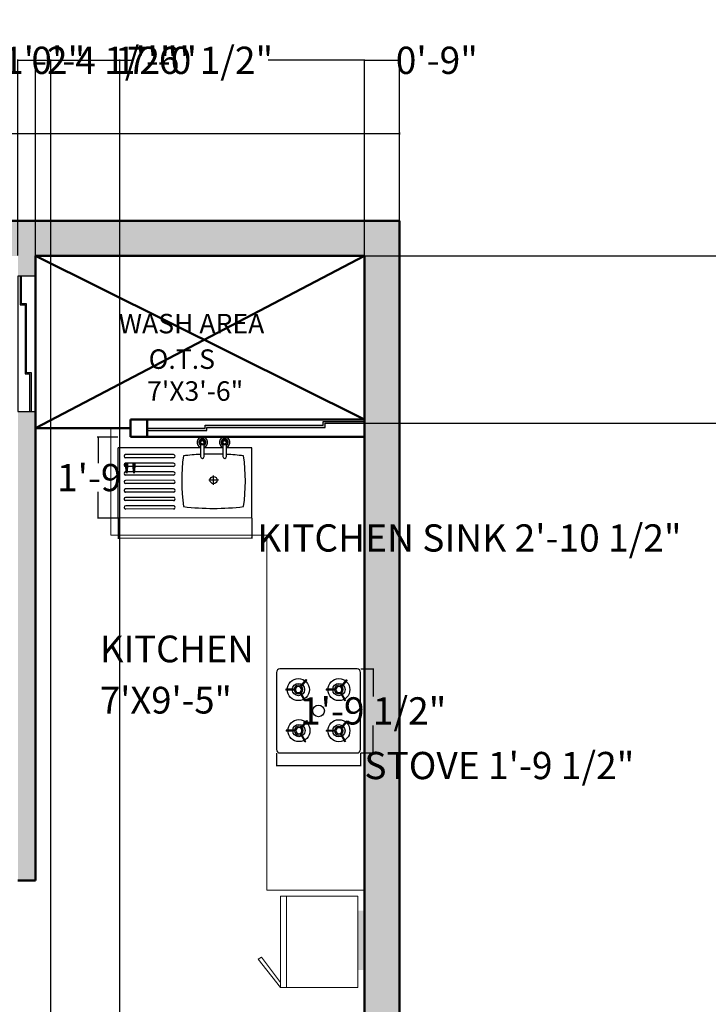
# Model space of a CAD drawing. Units: inches. Extents: x 48 to 822, y -191 to 651.
# Tile 8 of 13: x 268 to 445, y 398 to 651. Entities that reach past the tile are written whole.
import ezdxf

# ---------------------------------------------------------------- set-up
doc = ezdxf.new("R2010")
doc.units = ezdxf.units.IN
doc.header["$MEASUREMENT"] = 0
doc.layers.get('0').update_dxf_attribs({"color": 254})
for name, color, linetype, lineweight in [('A-ANNO-DIMS', 2, 'Continuous', 18), ('A-AREA-IDEN', 7, 'Continuous', 25), ('A-FLOR-FIXT', 8, 'Continuous', 18), ('A-FURN', 8, 'Continuous', 18), ('A-GLAZ', 4, 'Continuous', 25), ('A-WALL', 7, 'Continuous', 50), ('A-WALL-PATT', 8, 'Continuous', 13)]:
    doc.layers.add(name, color=color, linetype=linetype, lineweight=lineweight)
doc.layers.add('furniture', color=250, linetype='Continuous')
doc.styles.get("Standard").update_dxf_attribs({"font": 'arial.ttf'})
doc.dimstyles.get("Standard").update_dxf_attribs({"dimtxt": 7, "dimasz": 0.18, "dimexe": 0.18, "dimexo": 0.0625, "dimgap": 0.09, "dimtad": 0, "dimtih": 1, "dimtoh": 1, "dimzin": 0, "dimdsep": 46, "dimlunit": 3, "dimtxsty": 'Standard', "dimcen": 0.09, "dimadec": 0, "dimazin": 0, "dimtfac": 1, "dimtofl": 0, "dimtmove": 0, "dimatfit": 3, "dimfxl": 1, "dimtolj": 1, "dimtzin": 0, "dimarcsym": 0})

# ---------------------------------------------------------------- blocks, each defined once
blk = doc.blocks.new('4bstove')
at = {"layer": 'furniture'}
for p, q in [((1452.73, 1446.21), (1452.73, 1448.61)), ((1452.98, 1446.22), (1452.98, 1448.61)), ((1464.44, 1446.34), (1464.44, 1448.73)), ((1464.69, 1446.34), (1464.69, 1448.73)), ((1451.74, 1444.45), (1449.67, 1443.25)), ((1451.87, 1444.23), (1449.79, 1443.04)), ((1453.75, 1444.08), (1455.58, 1442.54)), ((1453.91, 1444.27), (1455.74, 1442.73)), ((1463.45, 1444.58), (1461.38, 1443.38)), ((1463.57, 1444.36), (1461.5, 1443.17)), ((1465.46, 1444.21), (1467.29, 1442.67)), ((1465.62, 1444.4), (1467.45, 1442.86)), ((1452.69, 1434.81), (1452.69, 1437.2)), ((1452.94, 1434.81), (1452.94, 1437.2)), ((1464.44, 1434.81), (1464.44, 1437.2)), ((1464.69, 1434.81), (1464.69, 1437.2)), ((1451.7, 1433.04), (1449.63, 1431.85)), ((1451.82, 1432.83), (1449.75, 1431.63)), ((1453.71, 1432.67), (1455.54, 1431.13)), ((1453.87, 1432.86), (1455.7, 1431.33)), ((1463.45, 1433.04), (1461.38, 1431.85)), ((1463.57, 1432.83), (1461.5, 1431.63)), ((1465.46, 1432.67), (1467.29, 1431.13)), ((1465.62, 1432.86), (1467.45, 1431.33))]:
    blk.add_line(p, q, dxfattribs=at)
for points in [[(1447.5, 1427.38), (1469.5, 1427.38, 0.414214), (1470.5, 1428.38), (1470.5, 1450.38, 0.414214), (1469.5, 1451.38), (1447.5, 1451.38, 0.414214), (1446.5, 1450.38), (1446.5, 1428.38, 0.414214)], [(1453.75, 1444.97, 1), (1452, 1444.97, 1)], [(1465.46, 1445.1, 1), (1463.71, 1445.1, 1)], [(1453.71, 1433.56, 1), (1451.96, 1433.56, 1)], [(1465.46, 1433.56, 1), (1463.71, 1433.56, 1)]]:
    blk.add_lwpolyline(points, format="xyb", close=True, dxfattribs=at)
for points in [[(1454.12, 1444.97, 1), (1451.62, 1444.97, 1), (1454.12, 1444.97, 1)], [(1465.83, 1445.1, 1), (1463.33, 1445.1, 1), (1465.83, 1445.1, 1)], [(1454.08, 1433.56, 1), (1451.58, 1433.56, 1), (1454.08, 1433.56, 1)], [(1465.83, 1433.56, 1), (1463.33, 1433.56, 1), (1465.83, 1433.56, 1)]]:
    blk.add_lwpolyline(points, format="xyb", dxfattribs=at)
for centre, radius in [((1452.87, 1444.97), 3.14), ((1464.58, 1445.1), 3.14), ((1452.87, 1444.97), 1.75), ((1464.58, 1445.1), 1.75), ((1458.5, 1439.38), 1.67), ((1452.83, 1433.56), 3.14), ((1464.58, 1433.56), 3.14), ((1452.83, 1433.56), 1.75), ((1464.58, 1433.56), 1.75)]:
    blk.add_circle(centre, radius, dxfattribs=at)
for centre, start, end in [((1452.87, 1444.97), 88.2645, 92.2039), ((1464.58, 1445.1), 88.2645, 92.2039), ((1452.87, 1444.97), 208.188, 212.1274), ((1452.87, 1444.97), 318.1018, 322.0412), ((1464.58, 1445.1), 208.188, 212.1274), ((1464.58, 1445.1), 318.1018, 322.0412), ((1452.83, 1433.56), 88.2645, 92.2039), ((1464.58, 1433.56), 88.2645, 92.2039)]:
    blk.add_arc(centre, 3.64, start, end, dxfattribs=at)
blk = doc.blocks.new('stove')
at = {"layer": 'furniture', "xscale": 0.9, "yscale": 0.9, "zscale": 0.9, "rotation": 89.99999999999999}
blk.add_blockref('4bstove', (1295.44, -1312.65), dxfattribs=at)
blk = doc.blocks.new('A$C799204C7')
for p, q in [((0, 34.2), (17.99, 34.2)), ((0, 0), (0, 34.2)), ((17.99, 13.08), (17.99, 34.2)), ((2.32, 20.01), (2.32, 32.27)), ((3.13, 20.01), (3.13, 32.27)), ((4.48, 20.01), (4.48, 32.27)), ((5.29, 20.01), (5.29, 32.27)), ((6.64, 20.01), (6.64, 32.27)), ((7.45, 20.01), (7.45, 32.27)), ((8.85, 20.01), (8.85, 32.27)), ((9.66, 20.01), (9.66, 32.27)), ((11.01, 20.01), (11.01, 32.27)), ((11.82, 20.01), (11.82, 32.27)), ((13.22, 20.01), (13.22, 32.27)), ((14.03, 20.01), (14.03, 32.27)), ((15.42, 20.01), (15.42, 32.27)), ((16.24, 20.01), (16.24, 32.27)), ((18.59, 13.08), (15.71, 13.08)), ((9.73, 11), (9.73, 8.54)), ((15.71, 12.17), (18.59, 12.17)), ((17.99, 7.36), (17.99, 12.17)), ((8.52, 9.77), (10.9, 9.77)), ((18.59, 7.36), (15.71, 7.36)), ((15.71, 6.45), (18.59, 6.45)), ((17.99, 0), (17.99, 6.45)), ((0, 0), (17.99, 0))]:
    blk.add_line(p, q)
for centre, radius in [((19.38, 12.62), 0.684), ((19.38, 12.62), 0.456), ((9.7, 9.77), 0.916), ((19.38, 6.91), 0.684), ((19.38, 6.91), 0.456)]:
    blk.add_circle(centre, radius)
for centre, radius, start, end in [((2.72, 32.27), 0.407, 0, 180), ((4.88, 32.27), 0.407, 0, 180), ((7.05, 32.27), 0.407, 0, 180), ((9.25, 32.27), 0.407, 0, 180), ((11.42, 32.27), 0.407, 0, 180), ((13.62, 32.27), 0.407, 0, 180), ((15.83, 32.27), 0.407, 0, 180), ((2.72, 20.01), 0.407, 180, 0), ((9.53, -30.19), 48.1, 82.3437, 97.8966), ((4.88, 20.01), 0.407, 180, 0), ((7.05, 20.01), 0.407, 180, 0), ((9.25, 20.01), 0.407, 180, 0), ((11.42, 20.01), 0.407, 180, 0), ((13.62, 20.01), 0.407, 180, 0), ((15.83, 20.01), 0.407, 180, 0), ((67.33, 9.77), 64.88, 173.1952, 186.8048), ((-48.51, 9.77), 64.88, 2.9208, 6.8048), ((15.71, 12.62), 0.456, 90, 270), ((19.38, 12.62), 1.37, 199.6514, 160.3603), ((19.38, 12.62), 0.911, 210.3431, 149.7554), ((-48.51, 9.77), 64.88, 357.8723, 2.115), ((19.38, 6.91), 1.37, 199.6514, 160.3603), ((19.38, 6.91), 0.911, 210.3431, 149.7554), ((15.71, 6.91), 0.456, 90, 270), ((-48.51, 9.77), 64.88, 353.1952, 357.0665), ((9.53, 49.73), 48.1, 262.1034, 277.6563)]:
    blk.add_arc(centre, radius, start, end)
blk = doc.blocks.new('sink')
at = {"layer": 'furniture'}
for p, q in [((8718164203.894819, -1433730582.369047), (8718164201.504578, -1433730582.369047)), ((8718164202.684322, -1433730581.131674), (8718164202.684322, -1433730583.598095)), ((8718164196.150837, -1433730592.638258), (8718164196.150837, -1433730604.938997)), ((8718164196.967728, -1433730592.638258), (8718164196.967728, -1433730604.938997)), ((8718164198.365185, -1433730592.638258), (8718164198.365185, -1433730604.938997)), ((8718164199.182076, -1433730592.638258), (8718164199.182076, -1433730604.938997)), ((8718164200.579533, -1433730592.638258), (8718164200.579533, -1433730604.938997)), ((8718164201.396423, -1433730592.638258), (8718164201.396423, -1433730604.938997)), ((8718164202.748692, -1433730592.638258), (8718164202.748692, -1433730604.938997)), ((8718164203.565582, -1433730592.638258), (8718164203.565582, -1433730604.938997)), ((8718164204.963041, -1433730592.638258), (8718164204.963041, -1433730604.938997)), ((8718164205.779934, -1433730592.638258), (8718164205.779934, -1433730604.938997)), ((8718164207.1322, -1433730592.638258), (8718164207.1322, -1433730604.938997)), ((8718164207.949093, -1433730592.638258), (8718164207.949093, -1433730604.938997)), ((8718164209.301359, -1433730592.638258), (8718164209.301359, -1433730604.938997)), ((8718164210.118252, -1433730592.638258), (8718164210.118252, -1433730604.938997))]:
    blk.add_line(p, q, dxfattribs=at)
for centre, radius in [((8718164192.998869, -1433730579.495552), 0.685789), ((8718164192.998869, -1433730579.495552), 0.457192), ((8718164202.715019, -1433730582.369047), 0.919003), ((8718164192.998869, -1433730585.228166), 0.68579), ((8718164192.998869, -1433730585.228166), 0.68579), ((8718164192.998869, -1433730585.228166), 0.457192)]:
    blk.add_circle(centre, radius, dxfattribs=at)
for centre, radius, start, end in [((8718164196.559284, -1433730592.638258), 0.41045, 354.3355999, 185.6644001), ((8718164198.77363, -1433730592.638258), 0.41045, 354.3355999, 185.6644001), ((8718164200.98798, -1433730592.638258), 0.41045, 354.3355999, 185.6644001), ((8718164203.157139, -1433730592.638258), 0.41045, 354.3355999, 185.6644001), ((8718164205.371487, -1433730592.638258), 0.41045, 354.3355999, 185.6644001), ((8718164207.540646, -1433730592.640262), 0.41045, 354.3355999, 185.6644001), ((8718164209.709805, -1433730592.640262), 0.41045, 354.3355999, 185.6644001), ((8718164196.559284, -1433730604.938997), 0.408445, 180, 0), ((8718164198.77363, -1433730604.938997), 0.408445, 180, 0), ((8718164200.98798, -1433730604.938997), 0.408445, 180, 0), ((8718164203.157139, -1433730604.938997), 0.408445, 180, 0), ((8718164205.371487, -1433730604.938997), 0.408445, 180, 0), ((8718164207.540646, -1433730604.938997), 0.408445, 180, 0), ((8718164209.709805, -1433730604.938997), 0.408445, 180, 0)]:
    blk.add_arc(centre, radius, start, end, dxfattribs=at)
at = {"layer": 'furniture', "xscale": 1.0032, "yscale": 1.0032, "zscale": 1.0032, "rotation": 180}
blk.add_blockref('A$C799204C7', (8718164212.441259, -1433730572.566334), dxfattribs=at)
blk = doc.blocks.new('washbasin')
at = {"layer": 'furniture'}
blk.add_blockref('sink', (-8718164214.119328, 1433730589.721069), dxfattribs=at)
blk = doc.blocks.new('*D16')
at = {"layer": 'A-ANNO-DIMS', "color": 0, "lineweight": -2, "transparency": 16777216}
for p, q in [((125.45, 622.39), (125.45, 621.91)), ((365.45, 622.39), (365.45, 621.91)), ((125.63, 622.09), (239.36, 622.09)), ((365.27, 622.09), (251.54, 622.09))]:
    blk.add_line(p, q, dxfattribs=at)
at = {"layer": 'A-ANNO-DIMS', "color": 0, "transparency": 16777216}
for points in [[(125.63, 622.12), (125.63, 622.06), (125.45, 622.09)], [(365.27, 622.12), (365.27, 622.06), (365.45, 622.09)]]:
    blk.add_solid(points, dxfattribs=at)
at = {"layer": 'Defpoints', "color": 0, "transparency": 16777216}
for p in [(125.45, 622.45), (365.45, 622.45), (365.45, 622.09)]:
    blk.add_point(p, dxfattribs=at)
at = {"layer": 'A-ANNO-DIMS', "color": 0, "transparency": 16777216, "insert": (245.45, 622.09), "char_height": 7, "attachment_point": 5}
blk.add_mtext("\\A1;20'", dxfattribs=at)
blk = doc.blocks.new('WIN-1500')
for p, q in [((300.62, 546.44), (315.51, 546.44)), ((315.51, 546.44), (315.51, 547.24)), ((315.51, 547.24), (345.84, 547.24)), ((315.95, 545.8), (315.95, 546.59)), ((315.95, 546.59), (346.31, 546.59)), ((345.84, 547.24), (345.84, 548.17)), ((345.84, 548.17), (356.45, 548.17)), ((346.31, 546.59), (346.31, 547.73)), ((346.31, 547.73), (356.45, 547.73)), ((300.62, 545.8), (315.95, 545.8))]:
    blk.add_line(p, q)
blk = doc.blocks.new('WIN-900-SLIT')
for p, q in [((271.95, 585.52), (267.45, 585.52)), ((267.45, 585.52), (267.45, 550.72)), ((268.05, 585.52), (268.05, 578.13)), ((268.38, 578.41), (268.38, 585.52)), ((271.95, 550.72), (271.95, 585.52)), ((268.05, 578.13), (269.28, 578.13)), ((269.63, 578.41), (268.38, 578.41)), ((269.28, 578.13), (269.28, 560.35)), ((269.63, 560.61), (269.63, 578.41)), ((269.28, 560.35), (270.46, 560.35)), ((270.92, 560.61), (269.63, 560.61)), ((270.46, 560.35), (270.46, 550.72)), ((270.92, 550.72), (270.92, 560.61)), ((267.45, 550.72), (271.95, 550.72))]:
    blk.add_line(p, q)
blk = doc.blocks.new('*D54')
at = {"layer": 'A-ANNO-DIMS', "color": 0, "lineweight": -2, "transparency": 16777216}
for p, q in [((333.84, 462.92), (333.84, 459.57)), ((355.44, 462.92), (355.44, 459.57)), ((334.02, 459.75), (355.26, 459.75)), ((355.44, 459.75), (355.62, 459.75))]:
    blk.add_line(p, q, dxfattribs=at)
at = {"layer": 'A-ANNO-DIMS', "color": 0, "transparency": 16777216}
for points in [[(334.02, 459.78), (334.02, 459.72), (333.84, 459.75)], [(355.26, 459.78), (355.26, 459.72), (355.44, 459.75)]]:
    blk.add_solid(points, dxfattribs=at)
at = {"layer": 'Defpoints', "color": 0, "transparency": 16777216}
for p in [(333.84, 462.99), (355.44, 462.99), (355.44, 459.75)]:
    blk.add_point(p, dxfattribs=at)
at = {"layer": 'A-ANNO-DIMS', "color": 0, "transparency": 16777216, "insert": (391.08, 459.75), "char_height": 7, "attachment_point": 5}
blk.add_mtext('\\A1;STOVE 1\'-9 1/2"', dxfattribs=at)
blk = doc.blocks.new('*D55')
at = {"layer": 'A-ANNO-DIMS', "color": 0, "lineweight": -2, "transparency": 16777216}
for p, q in [((355.5, 484.59), (358.86, 484.59)), ((358.68, 484.41), (358.68, 477.49)), ((358.68, 463.17), (358.68, 470.08)), ((355.5, 462.99), (358.86, 462.99))]:
    blk.add_line(p, q, dxfattribs=at)
at = {"layer": 'A-ANNO-DIMS', "color": 0, "transparency": 16777216}
for points in [[(358.65, 484.41), (358.71, 484.41), (358.68, 484.59)], [(358.65, 463.17), (358.71, 463.17), (358.68, 462.99)]]:
    blk.add_solid(points, dxfattribs=at)
at = {"layer": 'Defpoints', "color": 0, "transparency": 16777216}
for p in [(355.44, 484.59), (358.68, 484.59), (355.44, 462.99)]:
    blk.add_point(p, dxfattribs=at)
at = {"layer": 'A-ANNO-DIMS', "color": 0, "transparency": 16777216, "insert": (358.68, 473.79), "char_height": 7, "attachment_point": 5}
blk.add_mtext('\\A1;1\'-9 1/2"', dxfattribs=at)
blk = doc.blocks.new('*D58')
at = {"layer": 'A-ANNO-DIMS', "color": 0, "lineweight": -2, "transparency": 16777216}
for p, q in [((293.18, 523.27), (293.19, 518.01)), ((327.49, 523.3), (327.5, 518.04)), ((293.37, 518.19), (327.32, 518.22)), ((327.5, 518.22), (327.68, 518.22))]:
    blk.add_line(p, q, dxfattribs=at)
at = {"layer": 'A-ANNO-DIMS', "color": 0, "transparency": 16777216}
for points in [[(293.37, 518.22), (293.37, 518.16), (293.19, 518.19)], [(327.32, 518.25), (327.32, 518.19), (327.5, 518.22)]]:
    blk.add_solid(points, dxfattribs=at)
at = {"layer": 'Defpoints', "color": 0, "transparency": 16777216}
for p in [(293.18, 523.33), (327.49, 523.36), (327.5, 518.22)]:
    blk.add_point(p, dxfattribs=at)
at = {"layer": 'A-ANNO-DIMS', "color": 0, "transparency": 16777216, "insert": (383.38, 518.22), "char_height": 7, "attachment_point": 5}
blk.add_mtext('\\A1;KITCHEN SINK 2\'-10 1/2"', dxfattribs=at)
blk = doc.blocks.new('*D59')
at = {"layer": 'A-ANNO-DIMS', "color": 0, "lineweight": -2, "transparency": 16777216}
for p, q in [((293.1, 544.15), (287.84, 544.14)), ((288.02, 543.96), (288.03, 537.4)), ((288.04, 523.51), (288.03, 530.07)), ((293.12, 523.33), (287.86, 523.33))]:
    blk.add_line(p, q, dxfattribs=at)
at = {"layer": 'A-ANNO-DIMS', "color": 0, "transparency": 16777216}
for points in [[(288.05, 543.96), (287.99, 543.96), (288.02, 544.14)], [(288.07, 523.51), (288.01, 523.51), (288.04, 523.33)]]:
    blk.add_solid(points, dxfattribs=at)
at = {"layer": 'Defpoints', "color": 0, "transparency": 16777216}
for p in [(293.17, 544.15), (288.04, 523.33), (293.18, 523.33)]:
    blk.add_point(p, dxfattribs=at)
at = {"layer": 'A-ANNO-DIMS', "color": 0, "transparency": 16777216, "insert": (288.03, 533.73), "char_height": 7, "attachment_point": 5}
blk.add_mtext('\\A1;1\'-9"', dxfattribs=at)
blk = doc.blocks.new('*D62')
at = {"layer": 'A-ANNO-DIMS', "color": 0, "lineweight": -2, "transparency": 16777216}
for p, q in [((267.45, 590.75), (267.45, 641.12)), ((267.63, 640.94), (271.77, 640.94)), ((271.95, 590.75), (271.95, 641.12)), ((271.95, 640.94), (272.13, 640.94))]:
    blk.add_line(p, q, dxfattribs=at)
at = {"layer": 'A-ANNO-DIMS', "color": 0, "transparency": 16777216}
for points in [[(267.63, 640.97), (267.63, 640.91), (267.45, 640.94)], [(271.77, 640.97), (271.77, 640.91), (271.95, 640.94)]]:
    blk.add_solid(points, dxfattribs=at)
at = {"layer": 'Defpoints', "color": 0, "transparency": 16777216}
for p in [(271.95, 640.94), (267.45, 590.69), (271.95, 590.69)]:
    blk.add_point(p, dxfattribs=at)
at = {"layer": 'A-ANNO-DIMS', "color": 0, "transparency": 16777216, "insert": (289.68, 640.94), "char_height": 7, "attachment_point": 5}
blk.add_mtext('\\A1;0\'-4 1/2"', dxfattribs=at)
blk = doc.blocks.new('*D63')
at = {"layer": 'A-ANNO-DIMS', "color": 0, "lineweight": -2, "transparency": 16777216}
for p, q in [((271.95, 590.75), (271.95, 641.12)), ((272.13, 640.94), (296.68, 640.94)), ((356.27, 640.94), (331.72, 640.94)), ((356.45, 590.75), (356.45, 641.12))]:
    blk.add_line(p, q, dxfattribs=at)
at = {"layer": 'A-ANNO-DIMS', "color": 0, "transparency": 16777216}
for points in [[(272.13, 640.97), (272.13, 640.91), (271.95, 640.94)], [(356.27, 640.97), (356.27, 640.91), (356.45, 640.94)]]:
    blk.add_solid(points, dxfattribs=at)
at = {"layer": 'Defpoints', "color": 0, "transparency": 16777216}
for p in [(356.45, 640.94), (271.95, 590.69), (356.45, 590.69)]:
    blk.add_point(p, dxfattribs=at)
at = {"layer": 'A-ANNO-DIMS', "color": 0, "transparency": 16777216, "insert": (314.2, 640.94), "char_height": 7, "attachment_point": 5}
blk.add_mtext('\\A1;7\'-0 1/2"', dxfattribs=at)
blk = doc.blocks.new('*D64')
at = {"layer": 'A-ANNO-DIMS', "color": 0, "lineweight": -2, "transparency": 16777216}
for p, q in [((356.45, 590.75), (356.45, 641.12)), ((356.63, 640.94), (365.27, 640.94)), ((365.45, 599.75), (365.45, 641.12)), ((365.45, 640.94), (365.63, 640.94))]:
    blk.add_line(p, q, dxfattribs=at)
at = {"layer": 'A-ANNO-DIMS', "color": 0, "transparency": 16777216}
for points in [[(356.63, 640.97), (356.63, 640.91), (356.45, 640.94)], [(365.27, 640.97), (365.27, 640.91), (365.45, 640.94)]]:
    blk.add_solid(points, dxfattribs=at)
at = {"layer": 'Defpoints', "color": 0, "transparency": 16777216}
for p in [(365.45, 640.94), (365.45, 599.69), (356.45, 590.69)]:
    blk.add_point(p, dxfattribs=at)
at = {"layer": 'A-ANNO-DIMS', "color": 0, "transparency": 16777216, "insert": (375.02, 640.94), "char_height": 7, "attachment_point": 5}
blk.add_mtext('\\A1;0\'-9"', dxfattribs=at)
blk = doc.blocks.new('*D84')
at = {"layer": 'A-ANNO-DIMS', "color": 0, "lineweight": -2, "transparency": 16777216}
for p, q in [((356.51, 590.69), (790.04, 590.69)), ((789.86, 590.51), (789.86, 572.87)), ((789.86, 547.91), (789.86, 565.54)), ((356.51, 547.73), (790.04, 547.73))]:
    blk.add_line(p, q, dxfattribs=at)
at = {"layer": 'A-ANNO-DIMS', "color": 0, "transparency": 16777216}
for points in [[(789.83, 590.51), (789.89, 590.51), (789.86, 590.69)], [(789.83, 547.91), (789.89, 547.91), (789.86, 547.73)]]:
    blk.add_solid(points, dxfattribs=at)
at = {"layer": 'Defpoints', "color": 0, "transparency": 16777216}
for p in [(356.45, 590.69), (356.45, 547.73), (789.86, 547.73)]:
    blk.add_point(p, dxfattribs=at)
at = {"layer": 'A-ANNO-DIMS', "color": 0, "transparency": 16777216, "insert": (789.86, 569.21), "char_height": 7, "attachment_point": 5}
blk.add_mtext('\\A1;3\'-7"', dxfattribs=at)
blk = doc.blocks.new('*D90')
at = {"layer": 'A-ANNO-DIMS', "color": 0, "lineweight": -2, "transparency": 16777216}
for p, q in [((250.94, 295.25), (250.94, 641.12)), ((251.12, 640.94), (264.75, 640.94)), ((264.93, 295.25), (264.93, 641.12)), ((264.93, 640.94), (265.11, 640.94))]:
    blk.add_line(p, q, dxfattribs=at)
at = {"layer": 'A-ANNO-DIMS', "color": 0, "transparency": 16777216}
for points in [[(251.12, 640.97), (251.12, 640.91), (250.94, 640.94)], [(264.75, 640.97), (264.75, 640.91), (264.93, 640.94)]]:
    blk.add_solid(points, dxfattribs=at)
at = {"layer": 'Defpoints', "color": 0, "transparency": 16777216}
for p in [(264.93, 640.94), (250.94, 295.19), (264.93, 295.19)]:
    blk.add_point(p, dxfattribs=at)
at = {"layer": 'A-ANNO-DIMS', "color": 0, "transparency": 16777216, "insert": (274.17, 640.94), "char_height": 7, "attachment_point": 5}
blk.add_mtext('\\A1;1\'-2"', dxfattribs=at)
blk = doc.blocks.new('*D92')
at = {"layer": 'A-ANNO-DIMS', "color": 0, "lineweight": -2, "transparency": 16777216}
for p, q in [((275.91, 79.24), (275.91, 641.12)), ((276.09, 640.94), (293.48, 640.94)), ((293.66, 79.24), (293.66, 641.12)), ((293.66, 640.94), (293.84, 640.94))]:
    blk.add_line(p, q, dxfattribs=at)
at = {"layer": 'A-ANNO-DIMS', "color": 0, "transparency": 16777216}
for points in [[(276.09, 640.97), (276.09, 640.91), (275.91, 640.94)], [(293.48, 640.97), (293.48, 640.91), (293.66, 640.94)]]:
    blk.add_solid(points, dxfattribs=at)
at = {"layer": 'Defpoints', "color": 0, "transparency": 16777216}
for p in [(293.66, 640.94), (275.91, 79.18), (293.66, 79.18)]:
    blk.add_point(p, dxfattribs=at)
at = {"layer": 'A-ANNO-DIMS', "color": 0, "transparency": 16777216, "insert": (302.9, 640.94), "char_height": 7, "attachment_point": 5}
blk.add_mtext('\\A1;1\'-6"', dxfattribs=at)

msp = doc.modelspace()

# ---------------------------------------------------------------- hatches: boundary and pattern name
at = {"layer": 'A-FURN'}
h = msp.add_hatch(color=256, dxfattribs=at)
h.dxf.hatch_style = 1
h.paths.add_polyline_path([(356.334, 422.439), (354.769, 422.439), (354.769, 407.208), (356.334, 407.208)])
at = {"layer": 'A-WALL-PATT'}
h = msp.add_hatch(color=256, dxfattribs=at)
h.dxf.hatch_style = 1
h.paths.add_polyline_path([(134.451, 590.687), (267.451, 590.687), (267.451, 585.522), (271.951, 585.522), (271.951, 590.687), (356.451, 590.687), (356.451, 83.687), (348.824, 83.687), (348.824, 74.687), (365.451, 74.687), (365.451, 599.687), (125.451, 599.687), (125.451, -67.813), (171.204, -67.813), (171.204, -58.813), (134.451, -58.813), (134.451, 79.187), (193.069, 79.187), (193.069, 83.687), (134.451, 83.687), (134.451, 430.187), (190.775, 430.187), (190.775, 434.687), (134.451, 434.687)])
h.paths.add_polyline_path([(271.951, 550.72), (267.451, 550.72), (267.451, 430.187), (271.951, 430.187)], flags=17)
h.paths.add_polyline_path([(230.951, 432.437), (226.451, 432.437), (226.451, 376.187), (156.909, 376.187), (156.909, 371.687), (164.451, 371.687), (164.451, 359.12), (168.951, 359.12), (168.951, 371.687), (226.451, 371.687), (226.451, 335.687), (230.951, 335.687)], flags=17)
h.paths.add_polyline_path([(168.951, 341.37), (164.451, 341.37), (164.451, 299.687), (134.451, 299.687), (134.451, 295.187), (230.951, 295.187), (230.951, 299.687), (168.951, 299.687)], flags=17)
h.paths.add_polyline_path([(275.909, 83.687), (271.451, 83.687), (245.975, 83.687), (245.975, 79.187), (271.451, 79.187), (271.451, 15.696), (275.951, 15.696), (275.951, 79.177), (275.909, 79.177)], flags=17)
h.paths.add_polyline_path([(275.951, -40.13), (271.451, -40.13), (271.451, -58.813), (227.03, -58.813), (227.03, -67.813), (275.951, -67.813)], flags=17)
h = msp.add_hatch(color=256, dxfattribs=at)
h.dxf.hatch_style = 1
h.paths.add_polyline_path([(268.379, 585.522), (268.046, 585.522), (268.046, 578.127), (269.281, 578.127), (269.281, 560.346), (270.462, 560.346), (270.462, 550.72), (270.919, 550.72), (270.919, 560.611), (269.63, 560.611), (269.63, 578.406), (268.379, 578.406)])
h.paths.add_polyline_path([(315.954, 546.588), (346.307, 546.588), (346.307, 547.726), (356.451, 547.726), (356.451, 548.166), (345.839, 548.166), (345.839, 547.241), (315.513, 547.241), (315.513, 546.437), (300.625, 546.437), (300.625, 545.795), (315.954, 545.795)])
h.paths.add_polyline_path([(651.539, 585.522), (651.206, 585.522), (651.206, 578.127), (652.441, 578.127), (652.441, 560.346), (653.621, 560.346), (653.621, 550.72), (654.078, 550.72), (654.078, 560.611), (652.789, 560.611), (652.789, 578.406), (651.539, 578.406)])
h.paths.add_polyline_path([(656.709, 147.578), (655.571, 147.578), (655.571, 157.721), (655.131, 157.721), (655.131, 147.109), (656.055, 147.109), (656.055, 116.783), (656.86, 116.783), (656.86, 101.895), (657.501, 101.895), (657.501, 117.224), (656.709, 117.224)])

# ---------------------------------------------------------------- linework, layer by layer
at = {"layer": 'A-FURN'}
for p, q in [((291.27, 546.437), (291.27, 518.901)), ((291.27, 518.901), (331.354, 518.901)), ((331.354, 518.901), (331.354, 427.733)), ((331.354, 427.733), (356.451, 427.733)), ((334.844, 402.719), (334.844, 426.183)), ((334.844, 426.183), (354.769, 426.183)), ((336.438, 402.719), (336.438, 426.183)), ((354.769, 426.183), (354.769, 402.719)), ((329.129, 409.981), (330.043, 410.52)), ((334.844, 402.719), (329.129, 409.981)), ((330.043, 410.52), (334.844, 404)), ((354.769, 402.719), (334.844, 402.719))]:
    msp.add_line(p, q, dxfattribs=at)
at = {"layer": 'A-WALL'}
for p, q in [((125.451, 599.687), (365.451, 599.687)), ((365.451, 599.687), (365.451, -120.313)), ((271.951, 430.187), (271.951, 590.687)), ((271.951, 590.687), (356.451, 590.687)), ((271.951, 590.687), (356.451, 548.687)), ((271.951, 546.437), (356.451, 590.687)), ((356.451, 590.687), (356.451, 83.687)), ((296.371, 546.437), (271.951, 546.437)), ((296.371, 548.687), (356.451, 548.687)), ((296.371, 548.687), (296.371, 544.187)), ((300.625, 548.687), (300.625, 544.187)), ((356.451, 548.687), (300.625, 548.687)), ((356.451, 544.187), (356.451, 548.687)), ((296.371, 544.187), (356.451, 544.187)), ((300.625, 544.187), (356.451, 544.187)), ((267.451, 430.187), (271.951, 430.187))]:
    msp.add_line(p, q, dxfattribs=at)

# ---------------------------------------------------------------- block references
at = {"layer": 'A-FLOR-FIXT', "rotation": 270.052267437799}
msp.add_blockref('washbasin', (310.341, 521.669), dxfattribs=at)
at = {"layer": 'A-FLOR-FIXT'}
msp.add_blockref('stove', (344.637, 473.785), dxfattribs=at)
at = {"layer": 'A-GLAZ'}
for name in ['WIN-900-SLIT', 'WIN-1500']:
    msp.add_blockref(name, (0, 0), dxfattribs=at)

# ---------------------------------------------------------------- texts
at = {"layer": 'A-AREA-IDEN'}
for s, height, p in [('WASH AREA', 5.0075, (293.324, 570.788)), ('O.T.S', 5.0075, (301.03, 561.665)), ('7\'X3\'-6"', 5.0075, (300.626, 553.461)), ('KITCHEN', 6.866, (288.524, 486.268)), ('7\'X9\'-5"', 6.866, (288.524, 473.109))]:
    msp.add_text(s, height=height, dxfattribs=at).set_placement(p)

# ---------------------------------------------------------------- dimensions: what is measured, and where the dimension line sits
at = {"layer": 'A-ANNO-DIMS'}
for base, p1, p2, override, picture, middle in [((271.951, 640.937), (267.451, 590.687), (271.951, 590.687), {"dimdec": 1, "dimlfac": 1, "dimrnd": 0, "dimzin": 1, "dimdsep": 46, "dimlunit": 4, "dimfrac": 2}, '*D62', (289.68, 640.937)), ((356.451, 640.937), (271.951, 590.687), (356.451, 590.687), {"dimdec": 1, "dimlfac": 1, "dimrnd": 0, "dimzin": 1, "dimdsep": 46, "dimlunit": 4, "dimfrac": 2}, '*D63', (314.201, 640.937)), ((264.927, 640.937), (250.942, 295.187), (264.927, 295.187), {"dimdec": 1, "dimlfac": 1, "dimrnd": 0, "dimzin": 1, "dimdsep": 46, "dimlunit": 4, "dimfrac": 2}, '*D90', (274.172, 640.937)), ((293.6592, 640.9365), (275.9088, 79.1772), (293.6592, 79.1772), {"dimdec": 1, "dimlfac": 1, "dimrnd": 0, "dimzin": 1, "dimdsep": 46, "dimlunit": 4, "dimfrac": 2}, '*D92', (302.9036, 640.9365)), ((365.451, 640.937), (356.451, 590.687), (365.451, 599.687), {"dimdec": 1, "dimlfac": 1, "dimrnd": 0, "dimzin": 1, "dimdsep": 46, "dimlunit": 4, "dimfrac": 2}, '*D64', (375.025, 640.937)), ((365.451, 622.093), (125.451, 622.45), (365.451, 622.45), {"dimclrd": 0, "dimclre": 0, "dimclrt": 0}, '*D16', (245.451, 622.093))]:
    dim = msp.add_linear_dim(base=base, p1=p1, p2=p2, dimstyle='Standard', override=override, dxfattribs=at)
    dim.commit()
    dim.dimension.update_dxf_attribs({"geometry": picture, "text_midpoint": middle})
for base, p1, p2, angle, picture, middle in [((789.86, 547.726), (356.451, 590.687), (356.451, 547.726), 90, '*D84', (789.86, 569.206)), ((288.039, 523.327), (293.166, 544.146), (293.185, 523.332), 270.05227, '*D59', (288.029, 533.734)), ((358.677, 484.585), (355.437, 462.985), (355.437, 484.585), 90, '*D55', (358.677, 473.785))]:
    dim = msp.add_linear_dim(base=base, p1=p1, p2=p2, angle=angle, dimstyle='Standard', override={"dimdec": 1, "dimlfac": 1, "dimrnd": 0, "dimzin": 1, "dimdsep": 46, "dimlunit": 4, "dimfrac": 2}, dxfattribs=at)
    dim.commit()
    dim.dimension.update_dxf_attribs({"geometry": picture, "text_midpoint": middle})
dim = msp.add_linear_dim(base=(327.499, 518.217), p1=(293.185, 523.332), p2=(327.494, 523.363), angle=0.05227, text='KITCHEN SINK <>', dimstyle='Standard', override={"dimdec": 1, "dimlfac": 1, "dimrnd": 0, "dimzin": 1, "dimdsep": 46, "dimlunit": 4, "dimfrac": 2}, dxfattribs=at)
dim.commit()
dim.dimension.update_dxf_attribs({"geometry": '*D58', "text_midpoint": (383.382, 518.217)})
dim = msp.add_linear_dim(base=(355.437, 459.745), p1=(333.837, 462.985), p2=(355.437, 462.985), text='STOVE <>', dimstyle='Standard', override={"dimdec": 1, "dimlfac": 1, "dimrnd": 0, "dimzin": 1, "dimdsep": 46, "dimlunit": 4, "dimfrac": 2}, dxfattribs=at)
dim.commit()
dim.dimension.update_dxf_attribs({"geometry": '*D54', "text_midpoint": (391.081, 459.745)})

doc.saveas('drawing.dxf')
